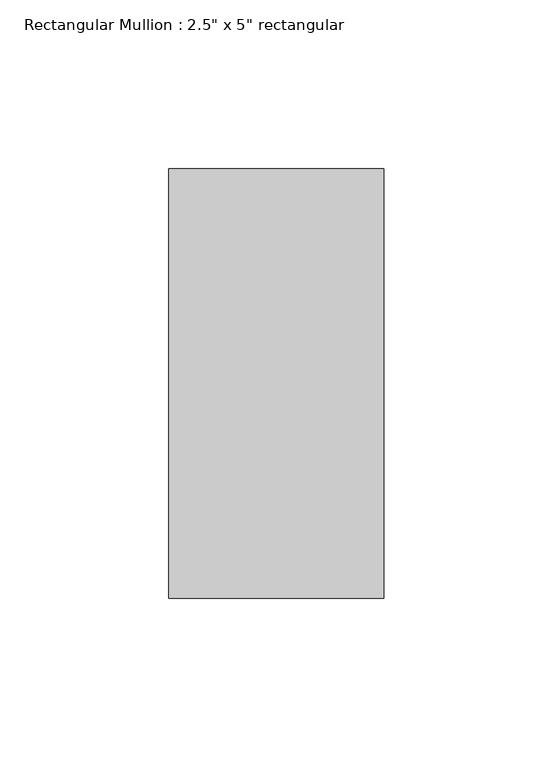
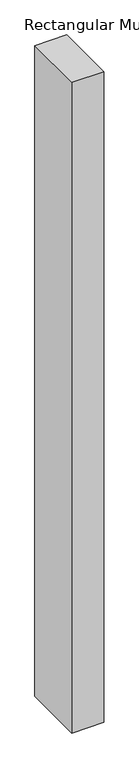
"""IFC4 building model written with IfcOpenShell, lengths in millimetres: member geometry."""

from ifc_helpers import new_model, si_unit, frame, origin, place, context, project, spatial, polyline, outline, extrude, source, transform, mapped, element, save


def member_0e93e1b1(model_context):
    return source(origin(), model_context, "Body", "SweptSolid", [
        extrude(outline(polyline([(0.0, 63.5), (0.0, -63.5), (-63.5, -63.5), (-63.5, 63.5), (0.0, 63.5)])), frame((0.0, 0.0, -1366.0685135), z_axis=(0.0, 0.0, 1.0), x_axis=(1.0, 0.0, 0.0)), (0.0, 0.0, 1.0), 1366.0685135),
    ])


if __name__ == "__main__":
    model = new_model("IFC4")
    model_context = context("Model", 3, world=origin())
    ifc_project = project(units=[si_unit("LENGTHUNIT", "METRE", prefix="MILLI")], contexts=[model_context])
    site = spatial("IfcSite", under=ifc_project)
    building = spatial("IfcBuilding", under=site)
    placement = place(None, origin())
    member_shape = member_0e93e1b1(model_context)
    element("IfcMember", 1, ObjectType="Rectangular Mullion : 2.5\" x 5\" rectangular", at=placement, inside=building, context=model_context, shape_type="MappedRepresentation", body=[
        mapped(member_shape, transform((0.0, 0.0, 0.0), x_axis=(1.0, 0.0, 0.0), y_axis=(0.0, 1.0, 0.0), z_axis=(0.0, 0.0, 1.0))),
    ])
    save(model, "model.ifc")

# Revit data of these elements
# Type "Rectangular Mullion : 2.5\" x 5\" rectangular"
#   built-in parameter 1007304 = 0.416667 (stored number, unit not read)
#   built-in parameter 1007301 = 0.104167 (stored number, unit not read)
#   built-in parameter 1007300 = 0.104167 (stored number, unit not read)
# Element 1 (IfcMember, "Rectangular Mullion : 2.5\" x 5\" rectangular")
#   Materials on its faces: "Aluminum"
# Materials
#   "Aluminum": class "Metal", colour RGB 247 247 247, transparency 0, Description = "Aluminum 6061", Cost = 0
